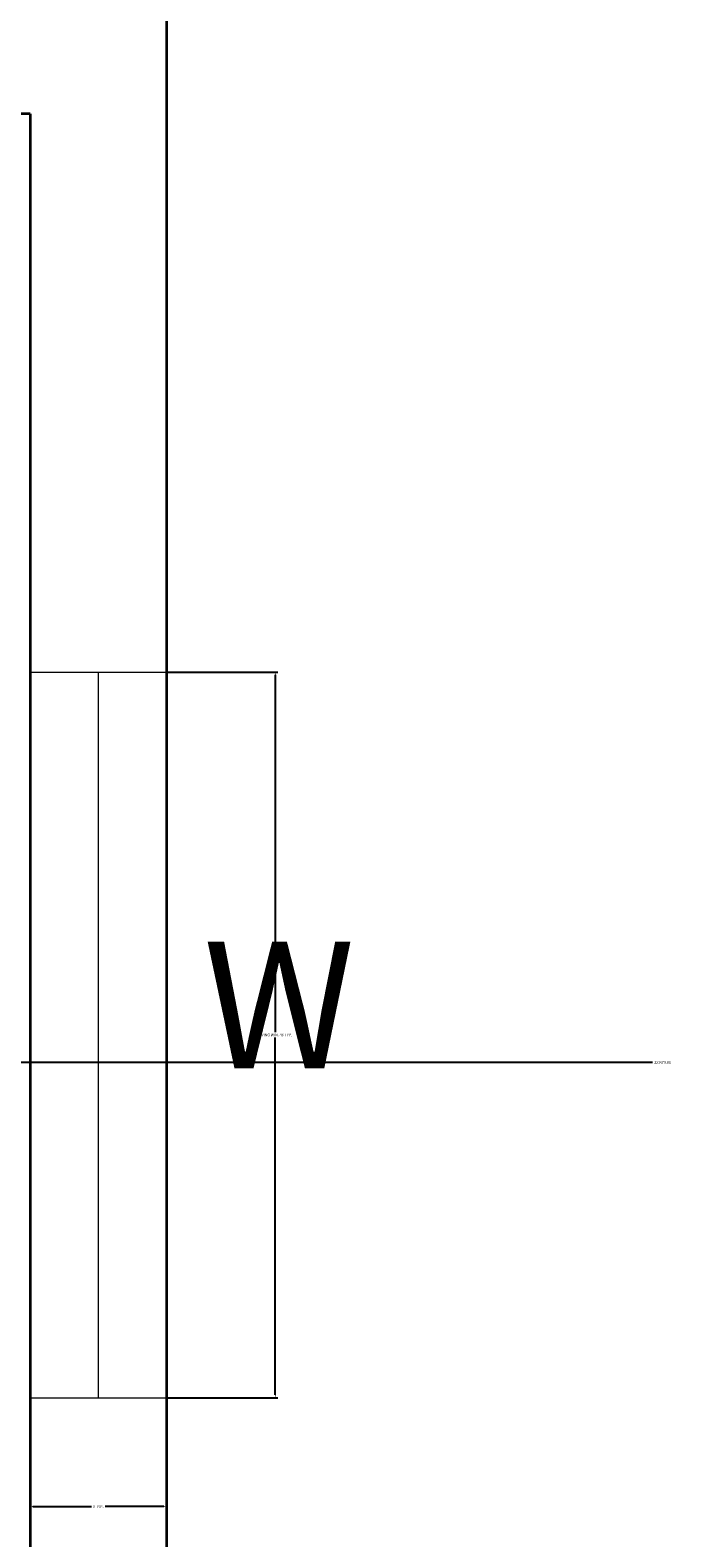
# Model space of a CAD drawing. Units: feet. Extents: x 1654 to 2985, y 1348 to 2230.
# Tile 52 of 53: x 2785 to 2827, y 1792 to 1892. Entities that reach past the tile are written whole.
import ezdxf

# ---------------------------------------------------------------- set-up
doc = ezdxf.new("R2010")
doc.units = ezdxf.units.FT
for name, color, linetype, lineweight in [('A-ANNO-DIMS', 2, 'Continuous', 18), ('A-ANNO-TEXT', 7, 'Continuous', 18), ('A-GLAZ', 4, 'Continuous', 18), ('A-WALL', 7, 'Continuous', 35)]:
    doc.layers.add(name, color=color, linetype=linetype, lineweight=lineweight)
doc.styles.get("Standard").update_dxf_attribs({"font": 'arial.ttf'})
doc.dimstyles.get("Standard").update_dxf_attribs({"dimtxt": 0.18, "dimasz": 0.18, "dimexe": 0.18, "dimexo": 0.0625, "dimgap": 0.09, "dimtad": 0, "dimtih": 1, "dimtoh": 1, "dimdec": 4, "dimzin": 0, "dimdsep": 46, "dimtxsty": 'Standard', "dimcen": 0.09, "dimadec": 0, "dimazin": 0, "dimtfac": 1, "dimtdec": 4, "dimtofl": 0, "dimtmove": 0, "dimatfit": 3, "dimfxl": 1, "dimtolj": 1, "dimtzin": 0, "dimarcsym": 0})

# ---------------------------------------------------------------- blocks, each defined once
blk = doc.blocks.new('WIN-LIVING-EAST')
for p, q in [((0, 47.934), (9, 47.934)), ((4.5, 47.934), (4.5, 0)), ((0, 0), (9, 0))]:
    blk.add_line(p, q)
blk = doc.blocks.new('*D62')
at = {"layer": 'A-ANNO-DIMS', "color": 0, "lineweight": -2, "transparency": 16777216}
for p, q in [((2793.768, 1849.371), (2801.076, 1849.371)), ((2800.896, 1849.191), (2800.896, 1825.587)), ((2800.896, 1801.617), (2800.896, 1825.221)), ((2793.768, 1801.437), (2801.076, 1801.437))]:
    blk.add_line(p, q, dxfattribs=at)
at = {"layer": 'A-ANNO-DIMS', "color": 0, "transparency": 16777216}
for points in [[(2800.866, 1849.191), (2800.926, 1849.191), (2800.896, 1849.371)], [(2800.866, 1801.617), (2800.926, 1801.617), (2800.896, 1801.437)]]:
    blk.add_solid(points, dxfattribs=at)
at = {"layer": 'Defpoints', "color": 0, "transparency": 16777216}
for p in [(2793.706, 1849.371), (2800.896, 1849.371), (2793.706, 1801.437)]:
    blk.add_point(p, dxfattribs=at)
at = {"layer": 'A-ANNO-DIMS', "color": 0, "transparency": 16777216, "insert": (2800.896, 1825.404), "char_height": 0.18, "attachment_point": 5}
blk.add_mtext('\\A1;LIVING WIN. 48 TYP.', dxfattribs=at)
blk = doc.blocks.new('*D63')
at = {"layer": 'A-ANNO-DIMS', "color": 0, "lineweight": -2, "transparency": 16777216}
for p, q in [((2784.706, 1801.375), (2784.706, 1794.067)), ((2793.706, 1801.375), (2793.706, 1794.067)), ((2784.886, 1794.247), (2788.748, 1794.247)), ((2793.526, 1794.247), (2789.664, 1794.247))]:
    blk.add_line(p, q, dxfattribs=at)
at = {"layer": 'A-ANNO-DIMS', "color": 0, "transparency": 16777216}
for points in [[(2784.886, 1794.277), (2784.886, 1794.217), (2784.706, 1794.247)], [(2793.526, 1794.277), (2793.526, 1794.217), (2793.706, 1794.247)]]:
    blk.add_solid(points, dxfattribs=at)
at = {"layer": 'Defpoints', "color": 0, "transparency": 16777216}
for p in [(2784.706, 1801.437), (2793.706, 1801.437), (2793.706, 1794.247)]:
    blk.add_point(p, dxfattribs=at)
at = {"layer": 'A-ANNO-DIMS', "color": 0, "transparency": 16777216, "insert": (2789.206, 1794.247), "char_height": 0.18, "attachment_point": 5}
blk.add_mtext('\\A1;9 TYP.', dxfattribs=at)
blk = doc.blocks.new('*D109')
at = {"layer": 'A-ANNO-DIMS', "color": 0, "lineweight": -2, "transparency": 16777216}
for p, q in [((2707.634, 1823.491), (2707.634, 1823.671)), ((2707.544, 1823.581), (2707.724, 1823.581)), ((2825.812, 1823.581), (2781.675, 1823.581))]:
    blk.add_line(p, q, dxfattribs=at)
at = {"layer": 'A-ANNO-DIMS', "color": 0, "transparency": 16777216}
blk.add_solid([(2781.675, 1823.611), (2781.675, 1823.551), (2781.495, 1823.581)], dxfattribs=at)
at = {"layer": 'Defpoints', "color": 0, "transparency": 16777216}
for p in [(2707.634, 1823.581), (2781.495, 1823.581)]:
    blk.add_point(p, dxfattribs=at)
at = {"layer": 'A-ANNO-DIMS', "color": 0, "transparency": 16777216, "insert": (2826.486, 1823.581), "char_height": 0.18, "attachment_point": 5}
blk.add_mtext('\\A1;2X R73.86', dxfattribs=at)

msp = doc.modelspace()

# ---------------------------------------------------------------- linework, layer by layer
at = {"layer": 'A-WALL'}
for p, q in [((2793.7058, 2117.2549), (2793.7058, 1742.2549)), ((2784.7058, 1886.2549), (2652.7058, 1886.2549)), ((2784.7058, 1886.2549), (2784.7058, 1751.2549)), ((2793.7058, 1886.2549), (2793.7058, 1523.2549))]:
    msp.add_line(p, q, dxfattribs=at)

# ---------------------------------------------------------------- block references
at = {"layer": 'A-GLAZ'}
msp.add_blockref('WIN-LIVING-EAST', (2784.7054, 1801.437), dxfattribs=at)

# ---------------------------------------------------------------- texts
at = {"layer": 'A-ANNO-TEXT'}
msp.add_text('W', height=8.3811, dxfattribs=at).set_placement((2796.1311, 1823.1912))

# ---------------------------------------------------------------- dimensions: what is measured, and where the dimension line sits
at = {"layer": 'A-ANNO-DIMS'}
dim = msp.add_linear_dim(base=(2800.8959, 1849.3712), p1=(2793.7058, 1801.4371), p2=(2793.7058, 1849.3712), angle=90, text='LIVING WIN. <> TYP.', dimstyle='Standard', override={"dimdec": 0, "dimlfac": 1, "dimrnd": 0, "dimzin": 0, "dimdsep": 46, "dimlunit": 2}, dxfattribs=at)
dim.commit()
dim.dimension.update_dxf_attribs({"geometry": '*D62', "text_midpoint": (2800.8959, 1825.4041)})
dim = msp.add_radius_dim(center=(2707.634, 1823.581), mpoint=(2781.495, 1823.581), text='2X <>', dimstyle='Standard', override={"dimdec": 2, "dimlfac": 1, "dimrnd": 0, "dimzin": 0, "dimdsep": 46, "dimlunit": 2}, dxfattribs=at)
dim.commit()
dim.dimension.update_dxf_attribs({"geometry": '*D109', "text_midpoint": (2825.8115, 1823.581), "dimtype": 164})
dim = msp.add_linear_dim(base=(2793.7058, 1794.2469), p1=(2784.7058, 1801.4371), p2=(2793.7058, 1801.4371), text='<> TYP.', dimstyle='Standard', override={"dimdec": 0, "dimlfac": 1, "dimrnd": 0, "dimzin": 0, "dimdsep": 46, "dimlunit": 2}, dxfattribs=at)
dim.commit()
dim.dimension.update_dxf_attribs({"geometry": '*D63', "text_midpoint": (2789.2058, 1794.2469)})

doc.saveas('drawing.dxf')
